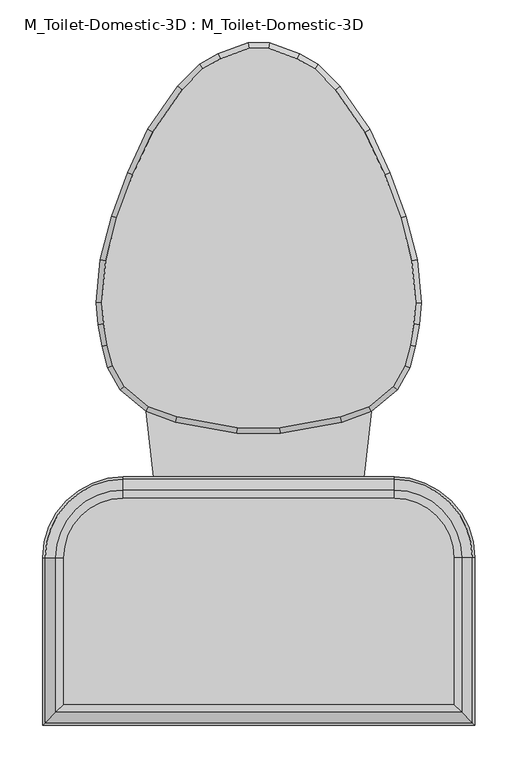
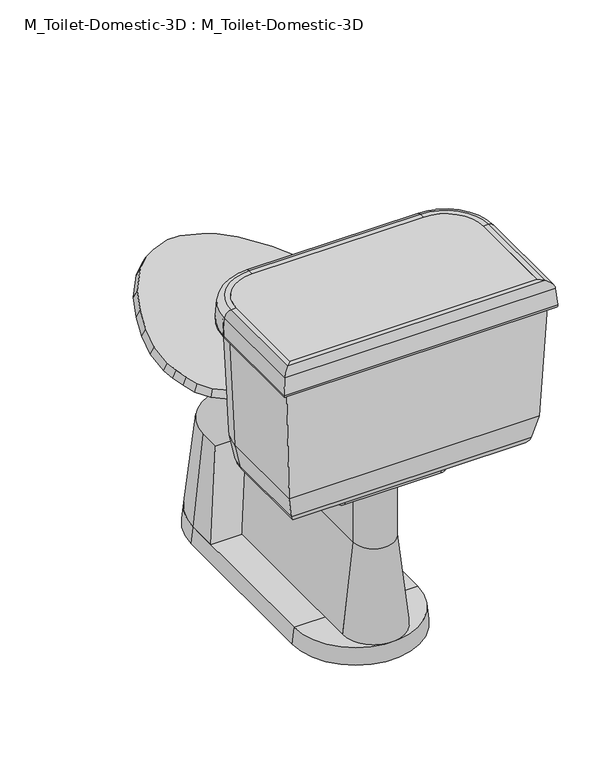
"""IFC4 building model written with IfcOpenShell, lengths in millimetres: flow terminal geometry, M_Toilet-Domestic-3D : M_Toilet-Domestic-3D."""

from ifc_helpers import new_model, si_unit, point, frame, frame_2d, origin, place, context, project, spatial, polyline, circle_curve, ellipse_curve, trimmed, segment, composite_curve, outline, extrude, faceted_brep, source, transform, mapped, element, save
from ifc_brep_helpers import plane_surface, cylinder_surface, revolved_surface, advanced_brep


def m_toilet_domestic_3d_m_toilet_domestic_3d_43425dfb(model_context):
    return source(origin(), model_context, "Body", "SolidModel", [
        advanced_brep(
        [(-117.7636364, -285.75, 0.0), (-114.3, -285.75, 31.75), (-38.1, -285.75, 31.75), (-38.1, -285.75, 0.0), (117.7636364, -285.75, 0.0), (38.1, -285.75, 0.0), (38.1, -285.75, 31.75), (114.3, -285.75, 31.75)],
        [
            (0, 1),
            (1, 2),
            (2, 3),
            (3, 0),
            (4, 5),
            (5, 6),
            (6, 7),
            (7, 4),
            (4, 0, circle_curve(frame((0.0, -285.75, 0.0), z_axis=(0.0, 0.0, -1.0), x_axis=(-1.0, 0.0, 0.0)), 117.7636364)),
            (3, 5, circle_curve(frame((0.0, -285.75, 0.0), z_axis=(0.0, 0.0, 1.0), x_axis=(-1.0, 0.0, 0.0)), 38.1)),
            (2, 6, circle_curve(frame((0.0, -285.75, 31.75), z_axis=(0.0, 0.0, 1.0), x_axis=(-1.0, 0.0, 0.0)), 38.1)),
            (1, 7, circle_curve(frame((0.0, -285.75, 31.75), z_axis=(0.0, 0.0, 1.0), x_axis=(-1.0, 0.0, 0.0)), 114.3)),
        ],
        [
            plane_surface(frame((0.0, -285.75, -304.8), z_axis=(0.0, 1.0, 0.0), x_axis=(-1.0, 0.0, 0.0))),
            plane_surface(frame((0.0, -285.75, -304.8), z_axis=(0.0, 1.0, 0.0), x_axis=(1.0, 0.0, 0.0))),
            plane_surface(frame((0.0, -285.75, 0.0), z_axis=(0.0, 0.0, -1.0), x_axis=(-1.0, 0.0, 0.0))),
            revolved_surface(polyline([(-38.1, -285.75, 0.0), (-38.1, -285.75, 31.75)]), (0.0, -285.75, -304.8), (0.0, 0.0, -1.0)),
            plane_surface(frame((0.0, -285.75, 31.75), z_axis=(0.0, 0.0, 1.0), x_axis=(-1.0, 0.0, 0.0))),
            revolved_surface(polyline([(-114.3, -285.75, 31.75), (-117.7636364, -285.75, 0.0)]), (0.0, -285.75, -304.8), (0.0, 0.0, -1.0)),
        ],
        [
            (0, [[1, 2, 3, 4]]),
            (1, [[5, 6, 7, 8]]),
            (2, [[-5, 9, -4, 10]]),
            (3, [[-6, -10, -3, 11]]),
            (4, [[-7, -11, -2, 12]]),
            (5, [[-8, -12, -1, -9]]),
        ],
    ),
        advanced_brep(
        [(-38.1, -342.9, 206.375), (-38.1, -342.9, 31.75), (-57.15, -342.9, 31.75), (38.1, -342.9, 206.375), (57.15, -342.9, 31.75), (38.1, -342.9, 31.75)],
        [
            (0, 1),
            (1, 2),
            (2, 0),
            (3, 4),
            (4, 5),
            (5, 3),
            (3, 0, circle_curve(frame((0.0, -342.9, 206.375), z_axis=(0.0, 0.0, -1.0), x_axis=(-1.0, 0.0, 0.0)), 38.1)),
            (2, 4, circle_curve(frame((0.0, -342.9, 31.75), z_axis=(0.0, 0.0, 1.0), x_axis=(-1.0, 0.0, 0.0)), 57.15)),
            (1, 5, circle_curve(frame((0.0, -342.9, 31.75), z_axis=(0.0, 0.0, 1.0), x_axis=(-1.0, 0.0, 0.0)), 38.1)),
        ],
        [
            plane_surface(frame((0.0, -342.9, 31.75), z_axis=(0.0, 1.0, 0.0), x_axis=(-1.0, 0.0, 0.0))),
            plane_surface(frame((0.0, -342.9, 31.75), z_axis=(0.0, 1.0, 0.0), x_axis=(1.0, 0.0, 0.0))),
            revolved_surface(polyline([(-38.1, -342.9, 206.375), (-57.15, -342.9, 31.75)]), (0.0, -342.9, 31.75), (0.0, 0.0, -1.0)),
            plane_surface(frame((0.0, -342.9, 31.75), z_axis=(0.0, 0.0, -1.0), x_axis=(-1.0, 0.0, 0.0))),
            revolved_surface(polyline([(-38.1, -342.9, 31.75), (-38.1, -342.9, 206.375)]), (0.0, -342.9, 31.75), (0.0, 0.0, -1.0)),
        ],
        [
            (0, [[1, 2, 3]]),
            (1, [[4, 5, 6]]),
            (2, [[-4, 7, -3, 8]]),
            (3, [[-5, -8, -2, 9]]),
            (4, [[-6, -9, -1, -7]]),
        ],
    ),
        faceted_brep([(-157.6293435, -97.472128, 400.05), (-129.0942628, -121.4159037, 400.05), (-95.7755003, -133.5429415, 400.05), (-24.844447, -146.05, 400.05), (24.844447, -146.05, 400.05), (95.7755003, -133.5429415, 400.05), (129.0942628, -121.4159037, 400.05), (157.6293435, -97.472128, 400.05), (171.060664, -73.773864, 400.05), (177.5851102, -49.4242991, 400.05), (181.9845715, -24.4737144, 400.05), (184.125744, 0.0, 400.05), (179.7950716, 49.4998127, 400.05), (166.347, 99.688699, 400.05), (148.0469602, 149.9676451, 400.05), (124.7045808, 200.0255393, 400.05), (90.0971582, 249.9125941, 400.05), (65.691017, 274.3187354, 400.05), (44.8990862, 286.3229622, 400.05), (11.5803237, 298.45, 400.05), (-11.5803237, 298.45, 400.05), (-44.8990862, 286.3229622, 400.05), (-65.691017, 274.3187354, 400.05), (-90.0971582, 249.9125941, 400.05), (-124.7045808, 200.0255393, 400.05), (-148.0469602, 149.9676451, 400.05), (-166.347, 99.688699, 400.05), (-179.7950716, 49.4998127, 400.05), (-184.125744, 0.0, 400.05), (-181.9845715, -24.4737144, 400.05), (-177.5851102, -49.4242991, 400.05), (-171.060664, -73.773864, 400.05), (-162.5887836, -101.6, 387.2181453), (-176.9845865, -76.2, 387.2181453), (-183.790496, -50.8, 387.2181453), (-188.2862441, -25.3033453, 387.2181453), (-190.5, 0.0, 387.2181453), (-186.0724883, 50.6066907, 387.2181453), (-172.4088722, 101.6, 387.2181453), (-153.9191843, 152.4, 387.2181453), (-130.2307553, 203.2, 387.2181453), (-94.9900085, 254.0, 387.2181453), (-69.5900085, 279.4, 387.2181453), (-47.5929632, 292.1, 387.2181453), (-12.7, 304.8, 387.2181453), (12.7, 304.8, 387.2181453), (47.5929632, 292.1, 387.2181453), (69.5900085, 279.4, 387.2181453), (94.9900085, 254.0, 387.2181453), (130.2307553, 203.2, 387.2181453), (153.9191843, 152.4, 387.2181453), (172.4088722, 101.6, 387.2181453), (186.0724883, 50.6066907, 387.2181453), (190.5, 0.0, 387.2181453), (188.2862441, -25.3033453, 387.2181453), (183.790496, -50.8, 387.2181453), (176.9845865, -76.2, 387.2181453), (162.5887836, -101.6, 387.2181453), (132.3182423, -127.0, 387.2181453), (97.4252791, -139.7, 387.2181453), (25.4, -152.4, 387.2181453), (-25.4, -152.4, 387.2181453), (-97.4252791, -139.7, 387.2181453), (-132.3182423, -127.0, 387.2181453)], [[[0, 1, 2, 3, 4, 5, 6, 7, 8, 9, 10, 11, 12, 13, 14, 15, 16, 17, 18, 19, 20, 21, 22, 23, 24, 25, 26, 27, 28, 29, 30, 31]], [[32, 33, 34, 35, 36, 37, 38, 39, 40, 41, 42, 43, 44, 45, 46, 47, 48, 49, 50, 51, 52, 53, 54, 55, 56, 57, 58, 59, 60, 61, 62, 63]], [[32, 0, 31, 33]], [[33, 31, 30, 34]], [[34, 30, 29, 35]], [[35, 29, 28, 36]], [[36, 28, 27, 37]], [[37, 27, 26, 38]], [[38, 26, 25, 39]], [[39, 25, 24, 40]], [[40, 24, 23, 41]], [[41, 23, 22, 42]], [[42, 22, 21, 43]], [[43, 21, 20, 44]], [[44, 20, 19, 45]], [[45, 19, 18, 46]], [[46, 18, 17, 47]], [[47, 17, 16, 48]], [[48, 16, 15, 49]], [[49, 15, 14, 50]], [[50, 14, 13, 51]], [[51, 13, 12, 52]], [[52, 12, 11, 53]], [[53, 11, 10, 54]], [[54, 10, 9, 55]], [[55, 9, 8, 56]], [[56, 8, 7, 57]], [[57, 7, 6, 58]], [[58, 6, 5, 59]], [[59, 5, 4, 60]], [[60, 4, 3, 61]], [[61, 3, 2, 62]], [[62, 2, 1, 63]], [[63, 1, 0, 32]]]),
        extrude(outline(composite_curve([segment(polyline([(228.5868869, -469.8868869), (-228.5868869, -469.8868869), (-228.5868869, -298.45)]), True, "CONTINUOUS"), segment(trimmed(circle_curve(frame_2d((-158.75, -298.45)), 69.8368869), [point((-228.5868869, -298.45))], [point((-158.75, -228.6131131))], False, "CARTESIAN"), True, "CONTINUOUS"), segment(polyline([(-158.75, -228.6131131), (158.75, -228.6131131)]), True, "CONTINUOUS"), segment(trimmed(circle_curve(frame_2d((158.75, -298.45)), 69.8368869), [point((158.75, -228.6131131))], [point((228.5868869, -298.45))], False, "CARTESIAN"), True, "CONTINUOUS"), segment(polyline([(228.5868869, -298.45), (228.5868869, -469.8868869)]), True, "CONTINUOUS")], self_intersect=False)), frame((0.0, 0.0, 654.05), z_axis=(0.0, 0.0, 1.0), x_axis=(1.0, 0.0, 0.0)), (0.0, 0.0, 1.0), 50.8),
        extrude(outline(composite_curve([segment(polyline([(-38.1, -342.9), (38.1, -342.9)]), True, "CONTINUOUS"), segment(trimmed(circle_curve(frame_2d((0.0, -342.9)), 38.1), [point((38.1, -342.9))], [point((-38.1, -342.9))], False, "CARTESIAN"), True, "CONTINUOUS")], self_intersect=False)), frame((0.0, 0.0, 206.375), z_axis=(0.0, 0.0, 1.0), x_axis=(1.0, 0.0, 0.0)), (0.0, 0.0, 1.0), 130.175),
        advanced_brep(
        [(177.8, -419.1, 387.2181453), (177.8, -298.45, 387.2181453), (177.8, -298.45, 374.65), (177.8, -419.1, 374.65), (192.8020829, -434.1020829, 387.2181453), (192.8020829, -298.45, 387.2181453), (211.4650931, -452.7650931, 402.4478636), (211.4650931, -298.45, 402.4478636), (218.7732506, -460.0732506, 438.15), (218.7732506, -298.45, 438.15), (228.5868869, -469.8868869, 654.05), (228.5868869, -298.45, 654.05), (228.5868869, -469.8868869, 704.85), (228.5868869, -298.45, 704.85), (237.91817, -479.21817, 704.85), (237.91817, -298.45, 704.85), (250.5698426, -491.8698426, 693.2568779), (250.5698426, -298.45, 693.2568779), (253.3960274, -494.6960274, 660.953439), (253.3960274, -298.45, 660.953439), (247.070191, -488.370191, 654.05), (247.070191, -298.45, 654.05), (241.3, -482.6, 654.05), (241.3, -298.45, 654.05), (231.4863636, -472.7863636, 438.15), (231.4863636, -298.45, 438.15), (222.3416824, -463.6416824, 393.4759963), (222.3416824, -298.45, 393.4759963), (197.8071664, -439.1071664, 374.65), (197.8071664, -298.45, 374.65), (158.75, -279.4, 387.2181453), (158.75, -279.4, 374.65), (158.75, -264.3979171, 387.2181453), (158.75, -245.7349069, 402.4478636), (158.75, -238.4267494, 438.15), (158.75, -228.6131131, 654.05), (158.75, -228.6131131, 704.85), (158.75, -219.28183, 704.85), (158.75, -206.6301574, 693.2568779), (158.75, -203.8039726, 660.953439), (158.75, -210.129809, 654.05), (158.75, -215.9, 654.05), (158.75, -225.7136364, 438.15), (158.75, -234.8583176, 393.4759963), (158.75, -259.3928336, 374.65), (-158.75, -279.4, 387.2181453), (-158.75, -279.4, 374.65), (-158.75, -264.3979171, 387.2181453), (-158.75, -245.7349069, 402.4478636), (-158.75, -238.4267494, 438.15), (-158.75, -228.6131131, 654.05), (-158.75, -228.6131131, 704.85), (-158.75, -219.28183, 704.85), (-158.75, -206.6301574, 693.2568779), (-158.75, -203.8039726, 660.953439), (-158.75, -210.129809, 654.05), (-158.75, -215.9, 654.05), (-158.75, -225.7136364, 438.15), (-158.75, -234.8583176, 393.4759963), (-158.75, -259.3928336, 374.65), (-177.8, -298.45, 387.2181453), (-177.8, -298.45, 374.65), (-192.8020829, -298.45, 387.2181453), (-211.4650931, -298.45, 402.4478636), (-218.7732506, -298.45, 438.15), (-228.5868869, -298.45, 654.05), (-228.5868869, -298.45, 704.85), (-237.91817, -298.45, 704.85), (-250.5698426, -298.45, 693.2568779), (-253.3960274, -298.45, 660.953439), (-247.070191, -298.45, 654.05), (-241.3, -298.45, 654.05), (-231.4863636, -298.45, 438.15), (-222.3416824, -298.45, 393.4759963), (-197.8071664, -298.45, 374.65), (-177.8, -419.1, 387.2181453), (-177.8, -419.1, 374.65), (-192.8020829, -434.1020829, 387.2181453), (-211.4650931, -452.7650931, 402.4478636), (-218.7732506, -460.0732506, 438.15), (-228.5868869, -469.8868869, 654.05), (-228.5868869, -469.8868869, 704.85), (-237.91817, -479.21817, 704.85), (-250.5698426, -491.8698426, 693.2568779), (-253.3960274, -494.6960274, 660.953439), (-247.070191, -488.370191, 654.05), (-241.3, -482.6, 654.05), (-231.4863636, -472.7863636, 438.15), (-222.3416824, -463.6416824, 393.4759963), (-197.8071664, -439.1071664, 374.65)],
        [
            (0, 1),
            (1, 2),
            (2, 3),
            (3, 0),
            (4, 5),
            (5, 1),
            (0, 4),
            (6, 7),
            (7, 5, circle_curve(frame((192.8020829, -298.45, 406.2681453), z_axis=(0.0, 1.0, 0.0), x_axis=(1.0, 0.0, 0.0)), 19.05)),
            (4, 6, ellipse_curve(frame((192.8020829, -434.1020829, 406.2681453), z_axis=(-0.7071067811865451, -0.7071067811865498, 0.0), x_axis=(-0.7071067811865497, 0.7071067811865452, 0.0)), 26.9407684, 19.05)),
            (8, 9),
            (9, 7),
            (6, 8),
            (10, 11),
            (11, 9),
            (8, 10),
            (12, 13),
            (13, 11),
            (10, 12),
            (14, 15),
            (15, 13),
            (12, 14),
            (16, 17),
            (17, 15, circle_curve(frame((237.91817, -298.45, 692.15), z_axis=(0.0, -1.0, 0.0), x_axis=(1.0, 0.0, 0.0)), 12.7)),
            (14, 16, ellipse_curve(frame((237.91817, -479.21817, 692.15), z_axis=(0.7071067811865451, 0.7071067811865498, 0.0), x_axis=(0.7071067811865497, -0.7071067811865452, 0.0)), 17.9605122, 12.7)),
            (18, 19),
            (19, 17),
            (16, 18),
            (20, 21),
            (21, 19, circle_curve(frame((247.070191, -298.45, 660.4), z_axis=(0.0, -1.0, 0.0), x_axis=(1.0, 0.0, 0.0)), 6.35)),
            (18, 20, ellipse_curve(frame((247.070191, -488.370191, 660.4), z_axis=(0.7071067811865451, 0.7071067811865498, 0.0), x_axis=(0.7071067811865497, -0.7071067811865452, 0.0)), 8.9802561, 6.35)),
            (22, 23),
            (23, 21),
            (20, 22),
            (24, 25),
            (25, 23),
            (22, 24),
            (26, 27),
            (27, 25),
            (24, 26),
            (28, 29),
            (29, 27, circle_curve(frame((197.8071664, -298.45, 400.05), z_axis=(0.0, -1.0, 0.0), x_axis=(1.0, 0.0, 0.0)), 25.4)),
            (26, 28, ellipse_curve(frame((197.8071664, -439.1071664, 400.05), z_axis=(0.7071067811865451, 0.7071067811865498, 0.0), x_axis=(0.7071067811865497, -0.7071067811865452, 0.0)), 35.9210245, 25.4)),
            (2, 29),
            (28, 3),
            (30, 31),
            (31, 2, circle_curve(frame((158.75, -298.45, 374.65), z_axis=(0.0, 0.0, -1.0), x_axis=(1.0, 0.0, 0.0)), 19.05)),
            (1, 30, circle_curve(frame((158.75, -298.45, 387.2181453), z_axis=(0.0, 0.0, 1.0), x_axis=(1.0, 0.0, 0.0)), 19.05)),
            (32, 30),
            (5, 32, circle_curve(frame((158.75, -298.45, 387.2181453), z_axis=(0.0, 0.0, 1.0), x_axis=(1.0, 0.0, 0.0)), 34.0520829)),
            (33, 32, circle_curve(frame((158.75, -264.3979171, 406.2681453), z_axis=(-1.0, 0.0, 0.0), x_axis=(0.0, 1.0, 0.0)), 19.05)),
            (7, 33, circle_curve(frame((158.75, -298.45, 402.4478636), z_axis=(0.0, 0.0, 1.0), x_axis=(1.0, 0.0, 0.0)), 52.7150931)),
            (34, 33),
            (9, 34, circle_curve(frame((158.75, -298.45, 438.15), z_axis=(0.0, 0.0, 1.0), x_axis=(1.0, 0.0, 0.0)), 60.0232506)),
            (35, 34),
            (11, 35, circle_curve(frame((158.75, -298.45, 654.05), z_axis=(0.0, 0.0, 1.0), x_axis=(1.0, 0.0, 0.0)), 69.8368869)),
            (36, 35),
            (13, 36, circle_curve(frame((158.75, -298.45, 704.85), z_axis=(0.0, 0.0, 1.0), x_axis=(1.0, 0.0, 0.0)), 69.8368869)),
            (37, 36),
            (15, 37, circle_curve(frame((158.75, -298.45, 704.85), z_axis=(0.0, 0.0, 1.0), x_axis=(1.0, 0.0, 0.0)), 79.16817)),
            (38, 37, circle_curve(frame((158.75, -219.28183, 692.15), z_axis=(1.0, 0.0, 0.0), x_axis=(0.0, 1.0, 0.0)), 12.7)),
            (17, 38, circle_curve(frame((158.75, -298.45, 693.2568779), z_axis=(0.0, 0.0, 1.0), x_axis=(1.0, 0.0, 0.0)), 91.8198426)),
            (39, 38),
            (19, 39, circle_curve(frame((158.75, -298.45, 660.953439), z_axis=(0.0, 0.0, 1.0), x_axis=(1.0, 0.0, 0.0)), 94.6460274)),
            (40, 39, circle_curve(frame((158.75, -210.129809, 660.4), z_axis=(1.0, 0.0, 0.0), x_axis=(0.0, 1.0, 0.0)), 6.35)),
            (21, 40, circle_curve(frame((158.75, -298.45, 654.05), z_axis=(0.0, 0.0, 1.0), x_axis=(1.0, 0.0, 0.0)), 88.320191)),
            (41, 40),
            (23, 41, circle_curve(frame((158.75, -298.45, 654.05), z_axis=(0.0, 0.0, 1.0), x_axis=(1.0, 0.0, 0.0)), 82.55)),
            (42, 41),
            (25, 42, circle_curve(frame((158.75, -298.45, 438.15), z_axis=(0.0, 0.0, 1.0), x_axis=(1.0, 0.0, 0.0)), 72.7363636)),
            (43, 42),
            (27, 43, circle_curve(frame((158.75, -298.45, 393.4759963), z_axis=(0.0, 0.0, 1.0), x_axis=(1.0, 0.0, 0.0)), 63.5916824)),
            (44, 43, circle_curve(frame((158.75, -259.3928336, 400.05), z_axis=(1.0, 0.0, 0.0), x_axis=(0.0, 1.0, 0.0)), 25.4)),
            (29, 44, circle_curve(frame((158.75, -298.45, 374.65), z_axis=(0.0, 0.0, 1.0), x_axis=(1.0, 0.0, 0.0)), 39.0571664)),
            (31, 44),
            (30, 45),
            (45, 46),
            (46, 31),
            (32, 47),
            (47, 45),
            (33, 48),
            (48, 47, circle_curve(frame((-158.75, -264.3979171, 406.2681453), z_axis=(-1.0, 0.0, 0.0), x_axis=(0.0, 1.0, 0.0)), 19.05)),
            (34, 49),
            (49, 48),
            (35, 50),
            (50, 49),
            (36, 51),
            (51, 50),
            (37, 52),
            (52, 51),
            (38, 53),
            (53, 52, circle_curve(frame((-158.75, -219.28183, 692.15), z_axis=(1.0, 0.0, 0.0), x_axis=(0.0, 1.0, 0.0)), 12.7)),
            (39, 54),
            (54, 53),
            (40, 55),
            (55, 54, circle_curve(frame((-158.75, -210.129809, 660.4), z_axis=(1.0, 0.0, 0.0), x_axis=(0.0, 1.0, 0.0)), 6.35)),
            (41, 56),
            (56, 55),
            (42, 57),
            (57, 56),
            (43, 58),
            (58, 57),
            (44, 59),
            (59, 58, circle_curve(frame((-158.75, -259.3928336, 400.05), z_axis=(1.0, 0.0, 0.0), x_axis=(0.0, 1.0, 0.0)), 25.4)),
            (46, 59),
            (60, 61),
            (61, 46, circle_curve(frame((-158.75, -298.45, 374.65), z_axis=(0.0, 0.0, -1.0), x_axis=(0.0, 1.0, 0.0)), 19.05)),
            (45, 60, circle_curve(frame((-158.75, -298.45, 387.2181453), z_axis=(0.0, 0.0, 1.0), x_axis=(0.0, 1.0, 0.0)), 19.05)),
            (62, 60),
            (47, 62, circle_curve(frame((-158.75, -298.45, 387.2181453), z_axis=(0.0, 0.0, 1.0), x_axis=(0.0, 1.0, 0.0)), 34.0520829)),
            (63, 62, circle_curve(frame((-192.8020829, -298.45, 406.2681453), z_axis=(0.0, -1.0, 0.0), x_axis=(-1.0, 0.0, 0.0)), 19.05)),
            (48, 63, circle_curve(frame((-158.75, -298.45, 402.4478636), z_axis=(0.0, 0.0, 1.0), x_axis=(0.0, 1.0, 0.0)), 52.7150931)),
            (64, 63),
            (49, 64, circle_curve(frame((-158.75, -298.45, 438.15), z_axis=(0.0, 0.0, 1.0), x_axis=(0.0, 1.0, 0.0)), 60.0232506)),
            (65, 64),
            (50, 65, circle_curve(frame((-158.75, -298.45, 654.05), z_axis=(0.0, 0.0, 1.0), x_axis=(0.0, 1.0, 0.0)), 69.8368869)),
            (66, 65),
            (51, 66, circle_curve(frame((-158.75, -298.45, 704.85), z_axis=(0.0, 0.0, 1.0), x_axis=(0.0, 1.0, 0.0)), 69.8368869)),
            (67, 66),
            (52, 67, circle_curve(frame((-158.75, -298.45, 704.85), z_axis=(0.0, 0.0, 1.0), x_axis=(0.0, 1.0, 0.0)), 79.16817)),
            (68, 67, circle_curve(frame((-237.91817, -298.45, 692.15), z_axis=(0.0, 1.0, 0.0), x_axis=(-1.0, 0.0, 0.0)), 12.7)),
            (53, 68, circle_curve(frame((-158.75, -298.45, 693.2568779), z_axis=(0.0, 0.0, 1.0), x_axis=(0.0, 1.0, 0.0)), 91.8198426)),
            (69, 68),
            (54, 69, circle_curve(frame((-158.75, -298.45, 660.953439), z_axis=(0.0, 0.0, 1.0), x_axis=(0.0, 1.0, 0.0)), 94.6460274)),
            (70, 69, circle_curve(frame((-247.070191, -298.45, 660.4), z_axis=(0.0, 1.0, 0.0), x_axis=(-1.0, 0.0, 0.0)), 6.35)),
            (55, 70, circle_curve(frame((-158.75, -298.45, 654.05), z_axis=(0.0, 0.0, 1.0), x_axis=(0.0, 1.0, 0.0)), 88.320191)),
            (71, 70),
            (56, 71, circle_curve(frame((-158.75, -298.45, 654.05), z_axis=(0.0, 0.0, 1.0), x_axis=(0.0, 1.0, 0.0)), 82.55)),
            (72, 71),
            (57, 72, circle_curve(frame((-158.75, -298.45, 438.15), z_axis=(0.0, 0.0, 1.0), x_axis=(0.0, 1.0, 0.0)), 72.7363636)),
            (73, 72),
            (58, 73, circle_curve(frame((-158.75, -298.45, 393.4759963), z_axis=(0.0, 0.0, 1.0), x_axis=(0.0, 1.0, 0.0)), 63.5916824)),
            (74, 73, circle_curve(frame((-197.8071664, -298.45, 400.05), z_axis=(0.0, 1.0, 0.0), x_axis=(-1.0, 0.0, 0.0)), 25.4)),
            (59, 74, circle_curve(frame((-158.75, -298.45, 374.65), z_axis=(0.0, 0.0, 1.0), x_axis=(0.0, 1.0, 0.0)), 39.0571664)),
            (61, 74),
            (60, 75),
            (75, 76),
            (76, 61),
            (62, 77),
            (77, 75),
            (63, 78),
            (78, 77, ellipse_curve(frame((-192.8020829, -434.1020829, 406.2681453), z_axis=(0.7071067811865498, -0.7071067811865451, 0.0), x_axis=(-0.7071067811865451, -0.70710678118655, 0.0)), 26.9407684, 19.05)),
            (64, 79),
            (79, 78),
            (65, 80),
            (80, 79),
            (66, 81),
            (81, 80),
            (67, 82),
            (82, 81),
            (68, 83),
            (83, 82, ellipse_curve(frame((-237.91817, -479.21817, 692.15), z_axis=(-0.7071067811865498, 0.7071067811865451, 0.0), x_axis=(0.7071067811865451, 0.70710678118655, 0.0)), 17.9605122, 12.7)),
            (69, 84),
            (84, 83),
            (70, 85),
            (85, 84, ellipse_curve(frame((-247.070191, -488.370191, 660.4), z_axis=(-0.7071067811865498, 0.7071067811865451, 0.0), x_axis=(0.7071067811865451, 0.70710678118655, 0.0)), 8.9802561, 6.35)),
            (71, 86),
            (86, 85),
            (72, 87),
            (87, 86),
            (73, 88),
            (88, 87),
            (74, 89),
            (89, 88, ellipse_curve(frame((-197.8071664, -439.1071664, 400.05), z_axis=(-0.7071067811865498, 0.7071067811865451, 0.0), x_axis=(0.7071067811865451, 0.70710678118655, 0.0)), 35.9210245, 25.4)),
            (76, 89),
            (75, 0),
            (3, 76),
            (77, 4),
            (78, 6),
            (79, 8),
            (80, 10),
            (81, 12),
            (82, 14),
            (83, 16),
            (84, 18),
            (85, 20),
            (86, 22),
            (87, 24),
            (88, 26),
            (89, 28),
        ],
        [
            plane_surface(frame((177.8, -419.1, 374.65), z_axis=(-1.0, 0.0, 0.0), x_axis=(0.0, 1.0, 0.0))),
            plane_surface(frame((177.8, -419.1, 387.2181453), z_axis=(0.0, 0.0, 1.0), x_axis=(0.0, 1.0, 0.0))),
            revolved_surface(polyline([(211.8520829, -298.45, 406.2681453), (211.8520829, -453.1520829260162, 406.2681453)]), (192.8020829, -419.1, 406.2681453), (0.0, 1.0, 0.0)),
            plane_surface(frame((211.4650931, -452.7650931, 402.4478636), z_axis=(-0.9796855721787505, 0.0, 0.2005397209153197), x_axis=(0.0, 1.0, 0.0))),
            plane_surface(frame((218.7732506, -460.0732506, 438.15), z_axis=(-0.9989685402102993, 0.0, 0.04540766091865541), x_axis=(0.0, 1.0, 0.0))),
            plane_surface(frame((228.5868869, -469.8868869, 654.05), z_axis=(-1.0, 0.0, 0.0), x_axis=(0.0, 1.0, 0.0))),
            plane_surface(frame((228.5868869, -469.8868869, 704.85), z_axis=(0.0, 0.0, 1.0), x_axis=(0.0, 1.0, 0.0))),
            cylinder_surface(frame((237.91817, -419.1, 692.15), z_axis=(0.0, -1.0, 0.0), x_axis=(1.0, 0.0, 0.0)), 12.7),
            plane_surface(frame((250.5698426, -491.8698426, 693.2568779), z_axis=(0.9961946980917448, 0.0, 0.08715574274766702), x_axis=(0.0, 1.0, 0.0))),
            cylinder_surface(frame((247.070191, -419.1, 660.4), z_axis=(0.0, -1.0, 0.0), x_axis=(1.0, 0.0, 0.0)), 6.35),
            plane_surface(frame((247.070191, -488.370191, 654.05), z_axis=(0.0, 0.0, -1.0), x_axis=(0.0, 1.0, 0.0))),
            plane_surface(frame((241.3, -482.6, 654.05), z_axis=(0.9989685402102995, 0.0, -0.04540766091865437), x_axis=(0.0, 1.0, 0.0))),
            plane_surface(frame((231.4863636, -472.7863636, 438.15), z_axis=(0.9796855721787479, 0.0, -0.2005397209153326), x_axis=(0.0, 1.0, 0.0))),
            cylinder_surface(frame((197.8071664, -419.1, 400.05), z_axis=(0.0, -1.0, 0.0), x_axis=(1.0, 0.0, 0.0)), 25.4),
            plane_surface(frame((197.8071664, -439.1071664, 374.65), z_axis=(0.0, 0.0, -1.0), x_axis=(0.0, 1.0, 0.0))),
            revolved_surface(polyline([(177.8, -298.45, 374.65), (177.8, -298.45, 387.2181453)]), (158.75, -298.45, 0.0), (0.0, 0.0, -1.0)),
            plane_surface(frame((158.75, -298.45, 387.2181453), z_axis=(0.0, 0.0, 1.0), x_axis=(1.0, 0.0, 0.0))),
            revolved_surface(trimmed(ellipse_curve(frame((192.8020829, -298.45, 406.2681453), z_axis=(0.0, -1.0, 0.0), x_axis=(1.0, 0.0, 0.0)), 19.05, 19.05), [point((192.8020829, -298.45, 387.2181453))], [point((211.4650931, -298.45, 402.4478636))], True, "CARTESIAN"), (158.75, -298.45, 0.0), (0.0, 0.0, -1.0)),
            revolved_surface(polyline([(211.4650931, -298.45, 402.4478636), (218.7732506, -298.45, 438.15)]), (158.75, -298.45, 0.0), (0.0, 0.0, -1.0)),
            revolved_surface(polyline([(218.7732506, -298.45, 438.15), (228.5868869, -298.45, 654.05)]), (158.75, -298.45, 0.0), (0.0, 0.0, -1.0)),
            revolved_surface(polyline([(228.5868869, -298.45, 654.05), (228.5868869, -298.45, 704.85)]), (158.75, -298.45, 0.0), (0.0, 0.0, -1.0)),
            plane_surface(frame((158.75, -298.45, 704.85), z_axis=(0.0, 0.0, 1.0), x_axis=(1.0, 0.0, 0.0))),
            revolved_surface(trimmed(ellipse_curve(frame((237.91817, -298.45, 692.15), z_axis=(0.0, 1.0, 0.0), x_axis=(1.0, 0.0, 0.0)), 12.7, 12.7), [point((237.91817, -298.45, 704.85))], [point((250.5698426, -298.45, 693.2568779))], True, "CARTESIAN"), (158.75, -298.45, 0.0), (0.0, 0.0, -1.0)),
            revolved_surface(polyline([(250.5698426, -298.45, 693.2568779), (253.3960274, -298.45, 660.953439)]), (158.75, -298.45, 0.0), (0.0, 0.0, -1.0)),
            revolved_surface(trimmed(ellipse_curve(frame((247.070191, -298.45, 660.4), z_axis=(0.0, 1.0, 0.0), x_axis=(1.0, 0.0, 0.0)), 6.35, 6.35), [point((253.3960274, -298.45, 660.953439))], [point((247.070191, -298.45, 654.05))], True, "CARTESIAN"), (158.75, -298.45, 0.0), (0.0, 0.0, -1.0)),
            plane_surface(frame((158.75, -298.45, 654.05), z_axis=(0.0, 0.0, -1.0), x_axis=(1.0, 0.0, 0.0))),
            revolved_surface(polyline([(241.3, -298.45, 654.05), (231.4863636, -298.45, 438.15)]), (158.75, -298.45, 0.0), (0.0, 0.0, -1.0)),
            revolved_surface(polyline([(231.4863636, -298.45, 438.15), (222.3416824, -298.45, 393.4759963)]), (158.75, -298.45, 0.0), (0.0, 0.0, -1.0)),
            revolved_surface(trimmed(ellipse_curve(frame((197.8071664, -298.45, 400.05), z_axis=(0.0, 1.0, 0.0), x_axis=(1.0, 0.0, 0.0)), 25.4, 25.4), [point((222.3416824, -298.45, 393.4759963))], [point((197.8071664, -298.45, 374.65))], True, "CARTESIAN"), (158.75, -298.45, 0.0), (0.0, 0.0, -1.0)),
            plane_surface(frame((158.75, -298.45, 374.65), z_axis=(0.0, 0.0, -1.0), x_axis=(1.0, 0.0, 0.0))),
            plane_surface(frame((158.75, -279.4, 374.65), z_axis=(0.0, -1.0, 0.0), x_axis=(-1.0, 0.0, 0.0))),
            plane_surface(frame((158.75, -279.4, 387.2181453), z_axis=(0.0, 0.0, 1.0), x_axis=(-1.0, 0.0, 0.0))),
            revolved_surface(polyline([(-158.75, -245.34791709999996, 406.2681453), (158.75, -245.34791709999996, 406.2681453)]), (158.75, -264.3979171, 406.2681453), (-1.0, 0.0, 0.0)),
            plane_surface(frame((158.75, -245.7349069, 402.4478636), z_axis=(0.0, -0.9796855721787505, 0.2005397209153197), x_axis=(-1.0, 0.0, 0.0))),
            plane_surface(frame((158.75, -238.4267494, 438.15), z_axis=(0.0, -0.9989685402102993, 0.04540766091865541), x_axis=(-1.0, 0.0, 0.0))),
            plane_surface(frame((158.75, -228.6131131, 654.05), z_axis=(0.0, -1.0, 0.0), x_axis=(-1.0, 0.0, 0.0))),
            plane_surface(frame((158.75, -228.6131131, 704.85), z_axis=(0.0, 0.0, 1.0), x_axis=(-1.0, 0.0, 0.0))),
            cylinder_surface(frame((158.75, -219.28183, 692.15), z_axis=(1.0, 0.0, 0.0), x_axis=(0.0, 1.0, 0.0)), 12.7),
            plane_surface(frame((158.75, -206.6301574, 693.2568779), z_axis=(0.0, 0.9961946980917448, 0.08715574274766702), x_axis=(-1.0, 0.0, 0.0))),
            cylinder_surface(frame((158.75, -210.129809, 660.4), z_axis=(1.0, 0.0, 0.0), x_axis=(0.0, 1.0, 0.0)), 6.35),
            plane_surface(frame((158.75, -210.129809, 654.05), z_axis=(0.0, 0.0, -1.0), x_axis=(-1.0, 0.0, 0.0))),
            plane_surface(frame((158.75, -215.9, 654.05), z_axis=(0.0, 0.9989685402102995, -0.04540766091865437), x_axis=(-1.0, 0.0, 0.0))),
            plane_surface(frame((158.75, -225.7136364, 438.15), z_axis=(0.0, 0.9796855721787479, -0.2005397209153326), x_axis=(-1.0, 0.0, 0.0))),
            cylinder_surface(frame((158.75, -259.3928336, 400.05), z_axis=(1.0, 0.0, 0.0), x_axis=(0.0, 1.0, 0.0)), 25.4),
            plane_surface(frame((158.75, -259.3928336, 374.65), z_axis=(0.0, 0.0, -1.0), x_axis=(-1.0, 0.0, 0.0))),
            revolved_surface(polyline([(-158.75, -279.4, 374.65), (-158.75, -279.4, 387.2181453)]), (-158.75, -298.45, 0.0), (0.0, 0.0, -1.0)),
            plane_surface(frame((-158.75, -298.45, 387.2181453), z_axis=(0.0, 0.0, 1.0), x_axis=(0.0, 1.0, 0.0))),
            revolved_surface(trimmed(ellipse_curve(frame((-158.75, -264.3979171, 406.2681453), z_axis=(1.0, 0.0, 0.0), x_axis=(0.0, 1.0, 0.0)), 19.05, 19.05), [point((-158.75, -264.3979171, 387.2181453))], [point((-158.75, -245.7349069, 402.4478636))], True, "CARTESIAN"), (-158.75, -298.45, 0.0), (0.0, 0.0, -1.0)),
            revolved_surface(polyline([(-158.75, -245.7349069, 402.4478636), (-158.75, -238.4267494, 438.15)]), (-158.75, -298.45, 0.0), (0.0, 0.0, -1.0)),
            revolved_surface(polyline([(-158.75, -238.4267494, 438.15), (-158.75, -228.6131131, 654.05)]), (-158.75, -298.45, 0.0), (0.0, 0.0, -1.0)),
            revolved_surface(polyline([(-158.75, -228.6131131, 654.05), (-158.75, -228.6131131, 704.85)]), (-158.75, -298.45, 0.0), (0.0, 0.0, -1.0)),
            plane_surface(frame((-158.75, -298.45, 704.85), z_axis=(0.0, 0.0, 1.0), x_axis=(0.0, 1.0, 0.0))),
            revolved_surface(trimmed(ellipse_curve(frame((-158.75, -219.28183, 692.15), z_axis=(-1.0, 0.0, 0.0), x_axis=(0.0, 1.0, 0.0)), 12.7, 12.7), [point((-158.75, -219.28183, 704.85))], [point((-158.75, -206.6301574, 693.2568779))], True, "CARTESIAN"), (-158.75, -298.45, 0.0), (0.0, 0.0, -1.0)),
            revolved_surface(polyline([(-158.75, -206.6301574, 693.2568779), (-158.75, -203.8039726, 660.953439)]), (-158.75, -298.45, 0.0), (0.0, 0.0, -1.0)),
            revolved_surface(trimmed(ellipse_curve(frame((-158.75, -210.129809, 660.4), z_axis=(-1.0, 0.0, 0.0), x_axis=(0.0, 1.0, 0.0)), 6.35, 6.35), [point((-158.75, -203.8039726, 660.953439))], [point((-158.75, -210.129809, 654.05))], True, "CARTESIAN"), (-158.75, -298.45, 0.0), (0.0, 0.0, -1.0)),
            plane_surface(frame((-158.75, -298.45, 654.05), z_axis=(0.0, 0.0, -1.0), x_axis=(0.0, 1.0, 0.0))),
            revolved_surface(polyline([(-158.75, -215.9, 654.05), (-158.75, -225.7136364, 438.15)]), (-158.75, -298.45, 0.0), (0.0, 0.0, -1.0)),
            revolved_surface(polyline([(-158.75, -225.7136364, 438.15), (-158.75, -234.8583176, 393.4759963)]), (-158.75, -298.45, 0.0), (0.0, 0.0, -1.0)),
            revolved_surface(trimmed(ellipse_curve(frame((-158.75, -259.3928336, 400.05), z_axis=(-1.0, 0.0, 0.0), x_axis=(0.0, 1.0, 0.0)), 25.4, 25.4), [point((-158.75, -234.8583176, 393.4759963))], [point((-158.75, -259.3928336, 374.65))], True, "CARTESIAN"), (-158.75, -298.45, 0.0), (0.0, 0.0, -1.0)),
            plane_surface(frame((-158.75, -298.45, 374.65), z_axis=(0.0, 0.0, -1.0), x_axis=(0.0, 1.0, 0.0))),
            plane_surface(frame((-177.8, -298.45, 374.65), z_axis=(1.0, 0.0, 0.0), x_axis=(0.0, -1.0, 0.0))),
            plane_surface(frame((-177.8, -298.45, 387.2181453), z_axis=(0.0, 0.0, 1.0), x_axis=(0.0, -1.0, 0.0))),
            revolved_surface(polyline([(-211.8520829, -453.15208292601636, 406.2681453), (-211.8520829, -298.45, 406.2681453)]), (-192.8020829, -298.45, 406.2681453), (0.0, -1.0, 0.0)),
            plane_surface(frame((-211.4650931, -298.45, 402.4478636), z_axis=(0.9796855721787505, 0.0, 0.2005397209153197), x_axis=(0.0, -1.0, 0.0))),
            plane_surface(frame((-218.7732506, -298.45, 438.15), z_axis=(0.9989685402102993, 0.0, 0.04540766091865541), x_axis=(0.0, -1.0, 0.0))),
            plane_surface(frame((-228.5868869, -298.45, 654.05), z_axis=(1.0, 0.0, 0.0), x_axis=(0.0, -1.0, 0.0))),
            plane_surface(frame((-228.5868869, -298.45, 704.85), z_axis=(0.0, 0.0, 1.0), x_axis=(0.0, -1.0, 0.0))),
            cylinder_surface(frame((-237.91817, -298.45, 692.15), z_axis=(0.0, 1.0, 0.0), x_axis=(-1.0, 0.0, 0.0)), 12.7),
            plane_surface(frame((-250.5698426, -298.45, 693.2568779), z_axis=(-0.9961946980917448, 0.0, 0.08715574274766702), x_axis=(0.0, -1.0, 0.0))),
            cylinder_surface(frame((-247.070191, -298.45, 660.4), z_axis=(0.0, 1.0, 0.0), x_axis=(-1.0, 0.0, 0.0)), 6.35),
            plane_surface(frame((-247.070191, -298.45, 654.05), z_axis=(0.0, 0.0, -1.0), x_axis=(0.0, -1.0, 0.0))),
            plane_surface(frame((-241.3, -298.45, 654.05), z_axis=(-0.9989685402102995, 0.0, -0.04540766091865437), x_axis=(0.0, -1.0, 0.0))),
            plane_surface(frame((-231.4863636, -298.45, 438.15), z_axis=(-0.9796855721787479, 0.0, -0.2005397209153326), x_axis=(0.0, -1.0, 0.0))),
            cylinder_surface(frame((-197.8071664, -298.45, 400.05), z_axis=(0.0, 1.0, 0.0), x_axis=(-1.0, 0.0, 0.0)), 25.4),
            plane_surface(frame((-197.8071664, -298.45, 374.65), z_axis=(0.0, 0.0, -1.0), x_axis=(0.0, -1.0, 0.0))),
            plane_surface(frame((-177.8, -419.1, 374.65), z_axis=(0.0, 1.0, 0.0), x_axis=(1.0, 0.0, 0.0))),
            plane_surface(frame((-177.8, -419.1, 387.2181453), z_axis=(0.0, 0.0, 1.0), x_axis=(1.0, 0.0, 0.0))),
            revolved_surface(polyline([(211.85208292601635, -453.15208290000004, 406.2681453), (-211.85208292601618, -453.15208290000004, 406.2681453)]), (-177.8, -434.1020829, 406.2681453), (1.0, 0.0, 0.0)),
            plane_surface(frame((-211.4650931, -452.7650931, 402.4478636), z_axis=(0.0, 0.9796855721787505, 0.2005397209153197), x_axis=(1.0, 0.0, 0.0))),
            plane_surface(frame((-218.7732506, -460.0732506, 438.15), z_axis=(0.0, 0.9989685402102993, 0.04540766091865541), x_axis=(1.0, 0.0, 0.0))),
            plane_surface(frame((-228.5868869, -469.8868869, 654.05), z_axis=(0.0, 1.0, 0.0), x_axis=(1.0, 0.0, 0.0))),
            plane_surface(frame((-228.5868869, -469.8868869, 704.85), z_axis=(0.0, 0.0, 1.0), x_axis=(1.0, 0.0, 0.0))),
            cylinder_surface(frame((-177.8, -479.21817, 692.15), z_axis=(-1.0, 0.0, 0.0), x_axis=(0.0, -1.0, 0.0)), 12.7),
            plane_surface(frame((-250.5698426, -491.8698426, 693.2568779), z_axis=(0.0, -0.9961946980917448, 0.08715574274766702), x_axis=(1.0, 0.0, 0.0))),
            cylinder_surface(frame((-177.8, -488.370191, 660.4), z_axis=(-1.0, 0.0, 0.0), x_axis=(0.0, -1.0, 0.0)), 6.35),
            plane_surface(frame((-247.070191, -488.370191, 654.05), z_axis=(0.0, 0.0, -1.0), x_axis=(1.0, 0.0, 0.0))),
            plane_surface(frame((-241.3, -482.6, 654.05), z_axis=(0.0, -0.9989685402102995, -0.04540766091865437), x_axis=(1.0, 0.0, 0.0))),
            plane_surface(frame((-231.4863636, -472.7863636, 438.15), z_axis=(0.0, -0.9796855721787479, -0.2005397209153326), x_axis=(1.0, 0.0, 0.0))),
            cylinder_surface(frame((-177.8, -439.1071664, 400.05), z_axis=(-1.0, 0.0, 0.0), x_axis=(0.0, -1.0, 0.0)), 25.4),
            plane_surface(frame((-197.8071664, -439.1071664, 374.65), z_axis=(0.0, 0.0, -1.0), x_axis=(1.0, 0.0, 0.0))),
        ],
        [
            (0, [[1, 2, 3, 4]]),
            (1, [[5, 6, -1, 7]]),
            (2, [[8, 9, -5, 10]]),
            (3, [[11, 12, -8, 13]]),
            (4, [[14, 15, -11, 16]]),
            (5, [[17, 18, -14, 19]]),
            (6, [[20, 21, -17, 22]]),
            (7, [[23, 24, -20, 25]]),
            (8, [[26, 27, -23, 28]]),
            (9, [[29, 30, -26, 31]]),
            (10, [[32, 33, -29, 34]]),
            (11, [[35, 36, -32, 37]]),
            (12, [[38, 39, -35, 40]]),
            (13, [[41, 42, -38, 43]]),
            (14, [[-3, 44, -41, 45]]),
            (15, [[46, 47, -2, 48]]),
            (16, [[49, -48, -6, 50]]),
            (17, [[51, -50, -9, 52]]),
            (18, [[53, -52, -12, 54]]),
            (19, [[55, -54, -15, 56]]),
            (20, [[57, -56, -18, 58]]),
            (21, [[59, -58, -21, 60]]),
            (22, [[61, -60, -24, 62]]),
            (23, [[63, -62, -27, 64]]),
            (24, [[65, -64, -30, 66]]),
            (25, [[67, -66, -33, 68]]),
            (26, [[69, -68, -36, 70]]),
            (27, [[71, -70, -39, 72]]),
            (28, [[73, -72, -42, 74]]),
            (29, [[75, -74, -44, -47]]),
            (30, [[76, 77, 78, -46]]),
            (31, [[79, 80, -76, -49]]),
            (32, [[81, 82, -79, -51]]),
            (33, [[83, 84, -81, -53]]),
            (34, [[85, 86, -83, -55]]),
            (35, [[87, 88, -85, -57]]),
            (36, [[89, 90, -87, -59]]),
            (37, [[91, 92, -89, -61]]),
            (38, [[93, 94, -91, -63]]),
            (39, [[95, 96, -93, -65]]),
            (40, [[97, 98, -95, -67]]),
            (41, [[99, 100, -97, -69]]),
            (42, [[101, 102, -99, -71]]),
            (43, [[103, 104, -101, -73]]),
            (44, [[-78, 105, -103, -75]]),
            (45, [[106, 107, -77, 108]]),
            (46, [[109, -108, -80, 110]]),
            (47, [[111, -110, -82, 112]]),
            (48, [[113, -112, -84, 114]]),
            (49, [[115, -114, -86, 116]]),
            (50, [[117, -116, -88, 118]]),
            (51, [[119, -118, -90, 120]]),
            (52, [[121, -120, -92, 122]]),
            (53, [[123, -122, -94, 124]]),
            (54, [[125, -124, -96, 126]]),
            (55, [[127, -126, -98, 128]]),
            (56, [[129, -128, -100, 130]]),
            (57, [[131, -130, -102, 132]]),
            (58, [[133, -132, -104, 134]]),
            (59, [[135, -134, -105, -107]]),
            (60, [[136, 137, 138, -106]]),
            (61, [[139, 140, -136, -109]]),
            (62, [[141, 142, -139, -111]]),
            (63, [[143, 144, -141, -113]]),
            (64, [[145, 146, -143, -115]]),
            (65, [[147, 148, -145, -117]]),
            (66, [[149, 150, -147, -119]]),
            (67, [[151, 152, -149, -121]]),
            (68, [[153, 154, -151, -123]]),
            (69, [[155, 156, -153, -125]]),
            (70, [[157, 158, -155, -127]]),
            (71, [[159, 160, -157, -129]]),
            (72, [[161, 162, -159, -131]]),
            (73, [[163, 164, -161, -133]]),
            (74, [[-138, 165, -163, -135]]),
            (75, [[166, -4, 167, -137]]),
            (76, [[168, -7, -166, -140]]),
            (77, [[169, -10, -168, -142]]),
            (78, [[170, -13, -169, -144]]),
            (79, [[171, -16, -170, -146]]),
            (80, [[172, -19, -171, -148]]),
            (81, [[173, -22, -172, -150]]),
            (82, [[174, -25, -173, -152]]),
            (83, [[175, -28, -174, -154]]),
            (84, [[176, -31, -175, -156]]),
            (85, [[177, -34, -176, -158]]),
            (86, [[178, -37, -177, -160]]),
            (87, [[179, -40, -178, -162]]),
            (88, [[180, -43, -179, -164]]),
            (89, [[-167, -45, -180, -165]]),
        ],
    ),
        extrude(outline(composite_curve([segment(polyline([(-25.4, -152.4), (0.0, -152.4), (25.4, -152.4), (97.4252791, -139.7), (132.3182423, -127.0), (101.4824733, -395.1508638)]), True, "CONTINUOUS"), segment(trimmed(circle_curve(frame_2d((88.8656197, -393.7)), 12.7), [point((101.4824733, -395.1508638))], [point((88.8656197, -406.4))], False, "CARTESIAN"), True, "CONTINUOUS"), segment(polyline([(88.8656197, -406.4), (-88.8656197, -406.4)]), True, "CONTINUOUS"), segment(trimmed(circle_curve(frame_2d((-88.8656197, -393.7)), 12.7), [point((-88.8656197, -406.4))], [point((-101.4824733, -395.1508638))], False, "CARTESIAN"), True, "CONTINUOUS"), segment(polyline([(-101.4824733, -395.1508638), (-132.3182423, -127.0), (-97.4252791, -139.7), (-25.4, -152.4)]), True, "CONTINUOUS")], self_intersect=False)), frame((0.0, 0.0, 336.55), z_axis=(0.0, 0.0, 1.0), x_axis=(1.0, 0.0, 0.0)), (0.0, 0.0, 1.0), 25.4),
        extrude(outline(polyline([(-139.7, 264.5247209), (-127.0, 229.6317577), (-107.4852632, 206.375), (-342.9, 206.375), (-342.9, 336.55), (-152.4, 336.55), (-139.7, 264.5247209)])), frame((-38.1, 0.0, 0.0), z_axis=(1.0, 0.0, 0.0), x_axis=(0.0, 1.0, 0.0)), (0.0, 0.0, 1.0), 76.2),
        advanced_brep(
        [(-117.7636364, -285.75, 0.0), (-38.1, -285.75, 0.0), (-38.1, -285.75, 31.75), (-114.3, -285.75, 31.75), (-114.3, 38.0999951, 31.75), (-117.7636364, 38.0999951, 0.0), (-38.1, 38.0999951, 31.75), (-38.1, 38.0999951, 0.0), (114.2999707, 38.0999951, 31.75), (117.7636071, 38.0999951, 0.0), (38.0999707, 38.0999951, 31.75), (38.0999707, 38.0999951, 0.0), (117.7636071, -285.6681634, 0.0), (114.2999707, -285.6681634, 31.75), (38.0999707, -285.6681634, 31.75), (38.0999707, -285.6681634, 0.0)],
        [
            (0, 1),
            (1, 2),
            (2, 3),
            (3, 0),
            (3, 4),
            (4, 5),
            (5, 0),
            (2, 6),
            (6, 4),
            (1, 7),
            (7, 6),
            (5, 7),
            (8, 9),
            (9, 5, circle_curve(frame((-1.46e-05, 38.0999951, 0.0), z_axis=(0.0, 0.0, 1.0), x_axis=(-1.0, 0.0, 0.0)), 117.7636217)),
            (4, 8, circle_curve(frame((-1.46e-05, 38.0999951, 31.75), z_axis=(0.0, 0.0, -1.0), x_axis=(-1.0, 0.0, 0.0)), 114.2999854)),
            (10, 8),
            (6, 10, circle_curve(frame((-1.46e-05, 38.0999951, 31.75), z_axis=(0.0, 0.0, -1.0), x_axis=(-1.0, 0.0, 0.0)), 38.0999854)),
            (11, 10),
            (7, 11, circle_curve(frame((-1.46e-05, 38.0999951, 0.0), z_axis=(0.0, 0.0, -1.0), x_axis=(-1.0, 0.0, 0.0)), 38.0999854)),
            (9, 11),
            (12, 13),
            (13, 14),
            (14, 15),
            (15, 12),
            (8, 13),
            (12, 9),
            (10, 14),
            (11, 15),
        ],
        [
            plane_surface(frame((-196.85, -285.75, 0.0), z_axis=(0.0, -1.0, 0.0), x_axis=(0.0, 0.0, -1.0))),
            plane_surface(frame((-117.7636364, -285.75, 0.0), z_axis=(-0.9941021766079929, 0.0, 0.10844751017543448), x_axis=(0.0, 1.0, 0.0))),
            plane_surface(frame((-114.3, -285.75, 31.75), z_axis=(0.0, 0.0, 1.0), x_axis=(0.0, 1.0, 0.0))),
            plane_surface(frame((-38.1, -285.75, 31.75), z_axis=(1.0, 0.0, 0.0), x_axis=(0.0, 1.0, 0.0))),
            plane_surface(frame((-38.1, -285.75, 0.0), z_axis=(0.0, 0.0, -1.0), x_axis=(0.0, 1.0, 0.0))),
            revolved_surface(polyline([(-117.7636364, 38.0999951, 0.0), (-114.3, 38.0999951, 31.75)]), (-1.46e-05, 38.0999951, 0.0), (0.0, 0.0, 1.0)),
            plane_surface(frame((-1.46e-05, 38.0999951, 31.75), z_axis=(0.0, 0.0, 1.0), x_axis=(-1.0, 0.0, 0.0))),
            revolved_surface(polyline([(-38.1, 38.0999951, 31.75), (-38.1, 38.0999951, 0.0)]), (-1.46e-05, 38.0999951, 0.0), (0.0, 0.0, 1.0)),
            plane_surface(frame((-1.46e-05, 38.0999951, 0.0), z_axis=(0.0, 0.0, -1.0), x_axis=(-1.0, 0.0, 0.0))),
            plane_surface(frame((31.7499707, -285.6681634, 0.0), z_axis=(0.0, -1.0, 0.0), x_axis=(0.0, 0.0, 1.0))),
            plane_surface(frame((117.7636071, 38.0999951, 0.0), z_axis=(0.9941021766079929, 0.0, 0.10844751017543448), x_axis=(0.0, -1.0, 0.0))),
            plane_surface(frame((114.2999707, 38.0999951, 31.75), z_axis=(0.0, 0.0, 1.0), x_axis=(0.0, -1.0, 0.0))),
            plane_surface(frame((38.0999707, 38.0999951, 31.75), z_axis=(-1.0, 0.0, 0.0), x_axis=(0.0, -1.0, 0.0))),
            plane_surface(frame((38.0999707, 38.0999951, 0.0), z_axis=(0.0, 0.0, -1.0), x_axis=(0.0, -1.0, 0.0))),
        ],
        [
            (0, [[1, 2, 3, 4]]),
            (1, [[5, 6, 7, -4]]),
            (2, [[8, 9, -5, -3]]),
            (3, [[10, 11, -8, -2]]),
            (4, [[-7, 12, -10, -1]]),
            (5, [[13, 14, -6, 15]]),
            (6, [[16, -15, -9, 17]]),
            (7, [[18, -17, -11, 19]]),
            (8, [[20, -19, -12, -14]]),
            (9, [[21, 22, 23, 24]]),
            (10, [[25, -21, 26, -13]]),
            (11, [[27, -22, -25, -16]]),
            (12, [[28, -23, -27, -18]]),
            (13, [[-26, -24, -28, -20]]),
        ],
    ),
        advanced_brep(
        [(-57.15, -342.9, 31.75), (-38.1, -342.9, 31.75), (-38.1, -342.9, 206.375), (-38.1, 0.0, 206.375), (-57.15, -19.05, 31.75), (-38.1, 0.0, 31.75), (-95.25, 0.0, 206.375), (-114.3, -19.05, 31.75), (-95.25, 0.0, 31.75), (-95.25, 38.1, 206.375), (-114.3, 38.1, 31.75), (-95.25, 38.1, 31.75), (95.25, 38.1, 206.375), (114.3, 38.1, 31.75), (95.25, 38.1, 31.75), (95.25, 0.0, 206.375), (114.3, -19.05, 31.75), (95.25, 0.0, 31.75), (38.1, 0.0, 206.375), (57.15, -19.05, 31.75), (38.1, 0.0, 31.75), (57.15, -342.9, 31.75), (38.1, -342.9, 206.375), (38.1, -342.9, 31.75)],
        [
            (0, 1),
            (1, 2),
            (2, 0),
            (2, 3),
            (3, 4),
            (4, 0),
            (1, 5),
            (5, 3),
            (4, 5),
            (3, 6),
            (6, 7),
            (7, 4),
            (5, 8),
            (8, 6),
            (7, 8),
            (6, 9),
            (9, 10),
            (10, 7),
            (8, 11),
            (11, 9),
            (10, 11),
            (12, 13),
            (13, 10, circle_curve(frame((0.0, 38.1, 31.75), z_axis=(0.0, 0.0, 1.0), x_axis=(-1.0, 0.0, 0.0)), 114.3)),
            (9, 12, circle_curve(frame((0.0, 38.1, 206.375), z_axis=(0.0, 0.0, -1.0), x_axis=(-1.0, 0.0, 0.0)), 95.25)),
            (14, 12),
            (11, 14, circle_curve(frame((0.0, 38.1, 31.75), z_axis=(0.0, 0.0, -1.0), x_axis=(-1.0, 0.0, 0.0)), 95.25)),
            (13, 14),
            (12, 15),
            (15, 16),
            (16, 13),
            (14, 17),
            (17, 15),
            (16, 17),
            (15, 18),
            (18, 19),
            (19, 16),
            (17, 20),
            (20, 18),
            (19, 20),
            (21, 22),
            (22, 23),
            (23, 21),
            (18, 22),
            (21, 19),
            (20, 23),
        ],
        [
            plane_surface(frame((-244.475, -342.9, 0.0), z_axis=(0.0, -1.0, 0.0), x_axis=(0.0, 0.0, -1.0))),
            plane_surface(frame((-57.15, -342.9, 31.75), z_axis=(-0.9941021766079944, 0.0, 0.10844751017542063), x_axis=(0.0, 1.0, 0.0))),
            plane_surface(frame((-38.1, -342.9, 206.375), z_axis=(1.0, 0.0, 0.0), x_axis=(0.0, 1.0, 0.0))),
            plane_surface(frame((-38.1, -342.9, 31.75), z_axis=(0.0, 0.0, -1.0), x_axis=(0.0, 1.0, 0.0))),
            plane_surface(frame((-57.15, -19.05, 31.75), z_axis=(0.0, -0.9941021766079944, 0.10844751017542063), x_axis=(-1.0, 0.0, 0.0))),
            plane_surface(frame((-38.1, 0.0, 206.375), z_axis=(0.0, 1.0, 0.0), x_axis=(-1.0, 0.0, 0.0))),
            plane_surface(frame((-38.1, 0.0, 31.75), z_axis=(0.0, 0.0, -1.0), x_axis=(-1.0, 0.0, 0.0))),
            plane_surface(frame((-114.3, -19.05, 31.75), z_axis=(-0.9941021766079944, 0.0, 0.10844751017542063), x_axis=(0.0, 1.0, 0.0))),
            plane_surface(frame((-95.25, 0.0, 206.375), z_axis=(1.0, 0.0, 0.0), x_axis=(0.0, 1.0, 0.0))),
            plane_surface(frame((-95.25, 0.0, 31.75), z_axis=(0.0, 0.0, -1.0), x_axis=(0.0, 1.0, 0.0))),
            revolved_surface(polyline([(-114.3, 38.1, 31.75), (-95.25, 38.1, 206.375)]), (0.0, 38.1, 0.0), (0.0, 0.0, 1.0)),
            revolved_surface(polyline([(-95.25, 38.1, 206.375), (-95.25, 38.1, 31.75)]), (0.0, 38.1, 0.0), (0.0, 0.0, 1.0)),
            plane_surface(frame((0.0, 38.1, 31.75), z_axis=(0.0, 0.0, -1.0), x_axis=(-1.0, 0.0, 0.0))),
            plane_surface(frame((114.3, 38.1, 31.75), z_axis=(0.9941021766079944, 0.0, 0.10844751017542063), x_axis=(0.0, -1.0, 0.0))),
            plane_surface(frame((95.25, 38.1, 206.375), z_axis=(-1.0, 0.0, 0.0), x_axis=(0.0, -1.0, 0.0))),
            plane_surface(frame((95.25, 38.1, 31.75), z_axis=(0.0, 0.0, -1.0), x_axis=(0.0, -1.0, 0.0))),
            plane_surface(frame((114.3, -19.05, 31.75), z_axis=(0.0, -0.9941021766079944, 0.10844751017542063), x_axis=(-1.0, 0.0, 0.0))),
            plane_surface(frame((95.25, 0.0, 206.375), z_axis=(0.0, 1.0, 0.0), x_axis=(-1.0, 0.0, 0.0))),
            plane_surface(frame((95.25, 0.0, 31.75), z_axis=(0.0, 0.0, -1.0), x_axis=(-1.0, 0.0, 0.0))),
            plane_surface(frame((-168.275, -342.9, 0.0), z_axis=(0.0, -1.0, 0.0), x_axis=(0.0, 0.0, 1.0))),
            plane_surface(frame((57.15, -19.05, 31.75), z_axis=(0.9941021766079944, 0.0, 0.10844751017542063), x_axis=(0.0, -1.0, 0.0))),
            plane_surface(frame((38.1, 0.0, 206.375), z_axis=(-1.0, 0.0, 0.0), x_axis=(0.0, -1.0, 0.0))),
            plane_surface(frame((38.1, 0.0, 31.75), z_axis=(0.0, 0.0, -1.0), x_axis=(0.0, -1.0, 0.0))),
        ],
        [
            (0, [[1, 2, 3]]),
            (1, [[4, 5, 6, -3]]),
            (2, [[7, 8, -4, -2]]),
            (3, [[-6, 9, -7, -1]]),
            (4, [[10, 11, 12, -5]]),
            (5, [[13, 14, -10, -8]]),
            (6, [[-12, 15, -13, -9]]),
            (7, [[16, 17, 18, -11]]),
            (8, [[19, 20, -16, -14]]),
            (9, [[-18, 21, -19, -15]]),
            (10, [[22, 23, -17, 24]]),
            (11, [[25, -24, -20, 26]]),
            (12, [[27, -26, -21, -23]]),
            (13, [[28, 29, 30, -22]]),
            (14, [[31, 32, -28, -25]]),
            (15, [[-30, 33, -31, -27]]),
            (16, [[34, 35, 36, -29]]),
            (17, [[37, 38, -34, -32]]),
            (18, [[-36, 39, -37, -33]]),
            (19, [[40, 41, 42]]),
            (20, [[43, -40, 44, -35]]),
            (21, [[45, -41, -43, -38]]),
            (22, [[-44, -42, -45, -39]]),
        ],
    ),
    ])


if __name__ == "__main__":
    model = new_model("IFC4")
    model_context = context("Model", 3, world=origin())
    ifc_project = project(units=[si_unit("LENGTHUNIT", "METRE", prefix="MILLI")], contexts=[model_context])
    site = spatial("IfcSite", under=ifc_project)
    building = spatial("IfcBuilding", under=site)
    placement = place(None, origin())
    m_toilet_domestic_3d_m_toilet_domestic_3d_shape = m_toilet_domestic_3d_m_toilet_domestic_3d_43425dfb(model_context)
    element("IfcFlowTerminal", 1, ObjectType="M_Toilet-Domestic-3D : M_Toilet-Domestic-3D", at=placement, inside=building, context=model_context, shape_type="MappedRepresentation", body=[
        mapped(m_toilet_domestic_3d_m_toilet_domestic_3d_shape, transform((0.0, 0.0, 0.0), x_axis=(1.0, 0.0, 0.0), y_axis=(0.0, 1.0, 0.0), z_axis=(0.0, 0.0, 1.0))),
    ])
    save(model, "model.ifc")

# Revit data of these elements
# Type "M_Toilet-Domestic-3D : M_Toilet-Domestic-3D"
#   Bowl/Basin Material = Porcelain, Linen
#   Seat Material = Laminate, Linen, Matte
#   Default Elevation = 0
# Element 1 (IfcFlowTerminal, "M_Toilet-Domestic-3D : M_Toilet-Domestic-3D")
#   Materials on its faces: "Porcelain, Linen", "Laminate, Linen, Matte"
# Materials
#   "Porcelain, Linen": class "Ceramic", colour RGB 249 239 230, transparency 0, Description = "Porcelain, linen", Cost = 0
#   "Laminate, Linen, Matte": class "Plastic", colour RGB 249 239 230, transparency 0, Description = "Plastic Laminate - Linen, Matte", Cost = 0
